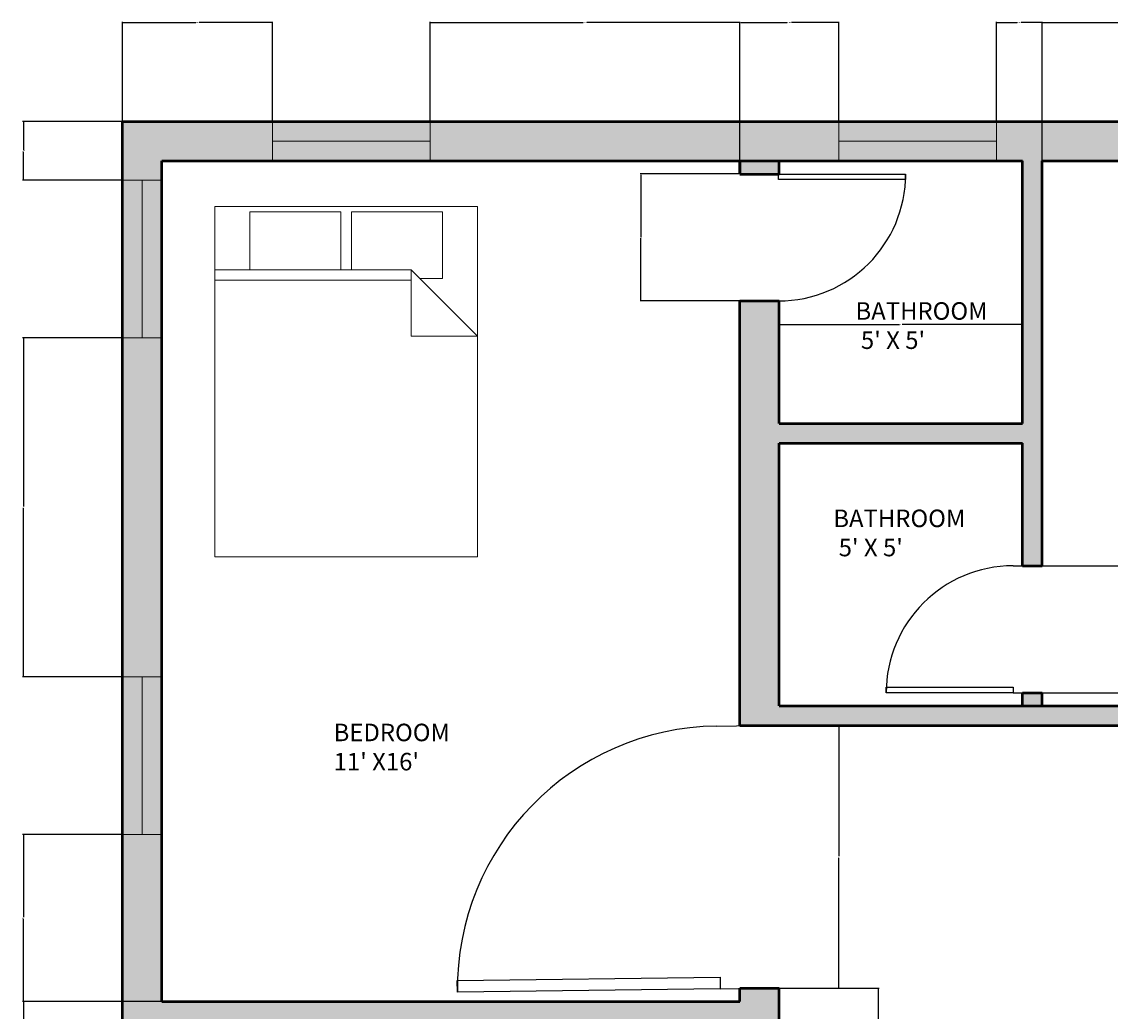
# Model space of a CAD drawing. Units: inches. Extents: x 7 to 493, y -11 to 454.
# Tile 2 of 4: x 7 to 255, y 228 to 454. Entities that reach past the tile are written whole.
import ezdxf

# ---------------------------------------------------------------- set-up
doc = ezdxf.new("R2010")
doc.units = ezdxf.units.IN
doc.header["$MEASUREMENT"] = 0
for name, color, linetype, lineweight in [('A-ANNO-DIMS', 2, 'Continuous', 18), ('A-AREA-IDEN', 7, 'Continuous', 25), ('A-WALL', 7, 'Continuous', 50), ('doors', 40, 'Continuous', 25), ('furniture', 220, 'Continuous', 18), ('window', 30, 'Continuous', 18)]:
    doc.layers.add(name, color=color, linetype=linetype, lineweight=lineweight)
doc.layers.add('A-WALL-PATT', color=251, linetype='Continuous', lineweight=13, true_color=0x636466)
doc.styles.get("Standard").update_dxf_attribs({"font": 'arial.ttf'})
doc.dimstyles.get("Standard").update_dxf_attribs({"dimtxt": 0.18, "dimasz": 0.18, "dimexe": 0.18, "dimexo": 0.0625, "dimgap": 0.09, "dimtad": 0, "dimtih": 1, "dimtoh": 1, "dimdec": 4, "dimzin": 0, "dimdsep": 46, "dimtxsty": 'Standard', "dimcen": 0.09, "dimadec": 0, "dimazin": 0, "dimtfac": 1, "dimtdec": 4, "dimtofl": 0, "dimtmove": 0, "dimatfit": 3, "dimfxl": 1, "dimtolj": 1, "dimtzin": 0, "dimarcsym": 0})

# ---------------------------------------------------------------- blocks, each defined once
blk = doc.blocks.new('Bed - Queen')
for p, q in [((0, -80.00003), (0, 0)), ((0, 0), (59.99999, 0)), ((59.99999, 0), (59.99999, -80.00003)), ((7.99999, -1.2), (28.79998, -1.2)), ((7.99999, -14.4), (7.99999, -1.2)), ((28.79998, -1.2), (28.79998, -14.4)), ((31.19999, -1.2), (51.99999, -1.2)), ((31.19999, -14.4), (31.19999, -1.2)), ((51.99999, -1.2), (51.99999, -16.4)), ((0, -14.4), (44.8, -14.4)), ((59.99999, -29.6), (44.8, -14.4)), ((44.8, -14.4), (44.8, -29.6)), ((44.8, -16.8), (0, -16.8)), ((51.99999, -16.4), (46.79936, -16.4)), ((44.8, -29.6), (59.99999, -29.6)), ((59.99999, -80.00003), (0, -80.00003))]:
    blk.add_line(p, q)
blk = doc.blocks.new('*U4')
for p, q in [((0, 0), (0, -6)), ((40, 0), (40, -6))]:
    blk.add_line(p, q)
blk.add_lwpolyline([(0, 0), (0, 40), (1.75, 40), (1.75, 0)], close=True)
blk.add_arc((0, 0), 40, 0, 90)
blk = doc.blocks.new('WIN-36IN')
for p, q in [((0, 0), (0, 9)), ((0, 9), (36, 9)), ((36, 9), (36, 0)), ((36, 9), (36, 4.5)), ((36, 4.5), (0, 4.5)), ((36, 0), (0, 0))]:
    blk.add_line(p, q)
blk = doc.blocks.new('*D24')
at = {"layer": 'A-ANNO-DIMS', "color": 0, "lineweight": -2, "transparency": 16777216}
for p, q in [((29.81, 431.55), (29.81, 454.27)), ((29.99, 454.09), (46.55, 454.09)), ((63.91, 454.09), (47.34, 454.09)), ((64.09, 431.55), (64.09, 454.27))]:
    blk.add_line(p, q, dxfattribs=at)
at = {"layer": 'A-ANNO-DIMS', "color": 0, "transparency": 16777216}
for points in [[(29.99, 454.12), (29.99, 454.06), (29.81, 454.09)], [(63.91, 454.12), (63.91, 454.06), (64.09, 454.09)]]:
    blk.add_solid(points, dxfattribs=at)
at = {"layer": 'Defpoints', "color": 0, "transparency": 16777216}
for p in [(64.09, 454.09), (29.81, 431.49), (64.09, 431.49)]:
    blk.add_point(p, dxfattribs=at)
at = {"layer": 'A-ANNO-DIMS', "color": 0, "transparency": 16777216, "insert": (46.95, 454.09), "char_height": 0.18, "attachment_point": 5}
blk.add_mtext('\\A1;34.28', dxfattribs=at)
blk = doc.blocks.new('*D25')
at = {"layer": 'A-ANNO-DIMS', "color": 0, "lineweight": -2, "transparency": 16777216}
for p, q in [((100.09, 431.55), (100.09, 454.27)), ((100.27, 454.09), (135.05, 454.09)), ((170.63, 454.09), (135.84, 454.09)), ((170.81, 422.55), (170.81, 454.27))]:
    blk.add_line(p, q, dxfattribs=at)
at = {"layer": 'A-ANNO-DIMS', "color": 0, "transparency": 16777216}
for points in [[(100.27, 454.12), (100.27, 454.06), (100.09, 454.09)], [(170.63, 454.12), (170.63, 454.06), (170.81, 454.09)]]:
    blk.add_solid(points, dxfattribs=at)
at = {"layer": 'Defpoints', "color": 0, "transparency": 16777216}
for p in [(170.81, 454.09), (100.09, 431.49), (170.81, 422.49)]:
    blk.add_point(p, dxfattribs=at)
at = {"layer": 'A-ANNO-DIMS', "color": 0, "transparency": 16777216, "insert": (135.45, 454.09), "char_height": 0.18, "attachment_point": 5}
blk.add_mtext('\\A1;70.72', dxfattribs=at)
blk = doc.blocks.new('*D26')
at = {"layer": 'A-ANNO-DIMS', "color": 0, "lineweight": -2, "transparency": 16777216}
for p, q in [((170.81, 422.55), (170.81, 454.27)), ((170.99, 454.09), (181.62, 454.09)), ((193.18, 454.09), (182.55, 454.09)), ((193.36, 431.55), (193.36, 454.27))]:
    blk.add_line(p, q, dxfattribs=at)
at = {"layer": 'A-ANNO-DIMS', "color": 0, "transparency": 16777216}
for points in [[(170.99, 454.12), (170.99, 454.06), (170.81, 454.09)], [(193.18, 454.12), (193.18, 454.06), (193.36, 454.09)]]:
    blk.add_solid(points, dxfattribs=at)
at = {"layer": 'Defpoints', "color": 0, "transparency": 16777216}
for p in [(193.36, 454.09), (193.36, 431.49), (170.81, 422.49)]:
    blk.add_point(p, dxfattribs=at)
at = {"layer": 'A-ANNO-DIMS', "color": 0, "transparency": 16777216, "insert": (182.08, 454.09), "char_height": 0.18, "attachment_point": 5}
blk.add_mtext('\\A1;22.553', dxfattribs=at)
blk = doc.blocks.new('*D27')
at = {"layer": 'A-ANNO-DIMS', "color": 0, "lineweight": -2, "transparency": 16777216}
for p, q in [((229.36, 431.55), (229.36, 454.27)), ((229.54, 454.09), (234.13, 454.09)), ((239.63, 454.09), (235.04, 454.09)), ((239.81, 422.55), (239.81, 454.27))]:
    blk.add_line(p, q, dxfattribs=at)
at = {"layer": 'A-ANNO-DIMS', "color": 0, "transparency": 16777216}
for points in [[(229.54, 454.12), (229.54, 454.06), (229.36, 454.09)], [(239.63, 454.12), (239.63, 454.06), (239.81, 454.09)]]:
    blk.add_solid(points, dxfattribs=at)
at = {"layer": 'Defpoints', "color": 0, "transparency": 16777216}
for p in [(239.81, 454.09), (229.36, 431.49), (239.81, 422.49)]:
    blk.add_point(p, dxfattribs=at)
at = {"layer": 'A-ANNO-DIMS', "color": 0, "transparency": 16777216, "insert": (234.58, 454.09), "char_height": 0.18, "attachment_point": 5}
blk.add_mtext('\\A1;10.447', dxfattribs=at)
blk = doc.blocks.new('*D28')
at = {"layer": 'A-ANNO-DIMS', "color": 0, "lineweight": -2, "transparency": 16777216}
for p, q in [((239.81, 422.55), (239.81, 454.27)), ((239.99, 454.09), (300.63, 454.09)), ((362.18, 454.09), (301.54, 454.09)), ((362.36, 431.55), (362.36, 454.27))]:
    blk.add_line(p, q, dxfattribs=at)
at = {"layer": 'A-ANNO-DIMS', "color": 0, "transparency": 16777216}
for points in [[(239.99, 454.12), (239.99, 454.06), (239.81, 454.09)], [(362.18, 454.12), (362.18, 454.06), (362.36, 454.09)]]:
    blk.add_solid(points, dxfattribs=at)
at = {"layer": 'Defpoints', "color": 0, "transparency": 16777216}
for p in [(362.36, 454.09), (362.36, 431.49), (239.81, 422.49)]:
    blk.add_point(p, dxfattribs=at)
at = {"layer": 'A-ANNO-DIMS', "color": 0, "transparency": 16777216, "insert": (301.08, 454.09), "char_height": 0.18, "attachment_point": 5}
blk.add_mtext('\\A1;122.55', dxfattribs=at)
blk = doc.blocks.new('*D33')
at = {"layer": 'A-ANNO-DIMS', "color": 0, "lineweight": -2, "transparency": 16777216}
for p, q in [((38.74, 230.49), (7.03, 230.49)), ((7.21, 230.31), (7.21, 216.31)), ((7.21, 201.94), (7.21, 215.94)), ((29.74, 201.76), (7.03, 201.76))]:
    blk.add_line(p, q, dxfattribs=at)
at = {"layer": 'A-ANNO-DIMS', "color": 0, "transparency": 16777216}
for points in [[(7.18, 230.31), (7.24, 230.31), (7.21, 230.49)], [(7.18, 201.94), (7.24, 201.94), (7.21, 201.76)]]:
    blk.add_solid(points, dxfattribs=at)
at = {"layer": 'Defpoints', "color": 0, "transparency": 16777216}
for p in [(7.21, 230.49), (38.81, 230.49), (29.81, 201.76)]:
    blk.add_point(p, dxfattribs=at)
at = {"layer": 'A-ANNO-DIMS', "color": 0, "transparency": 16777216, "insert": (7.21, 216.13), "char_height": 0.18, "attachment_point": 5}
blk.add_mtext('\\A1;28.72', dxfattribs=at)
blk = doc.blocks.new('*D34')
at = {"layer": 'A-ANNO-DIMS', "color": 0, "lineweight": -2, "transparency": 16777216}
for p, q in [((29.74, 268.63), (7.03, 268.63)), ((7.21, 268.45), (7.21, 249.74)), ((7.21, 230.67), (7.21, 249.37)), ((38.74, 230.49), (7.03, 230.49))]:
    blk.add_line(p, q, dxfattribs=at)
at = {"layer": 'A-ANNO-DIMS', "color": 0, "transparency": 16777216}
for points in [[(7.18, 268.45), (7.24, 268.45), (7.21, 268.63)], [(7.18, 230.67), (7.24, 230.67), (7.21, 230.49)]]:
    blk.add_solid(points, dxfattribs=at)
at = {"layer": 'Defpoints', "color": 0, "transparency": 16777216}
for p in [(7.21, 268.63), (29.81, 268.63), (38.81, 230.49)]:
    blk.add_point(p, dxfattribs=at)
at = {"layer": 'A-ANNO-DIMS', "color": 0, "transparency": 16777216, "insert": (7.21, 249.56), "char_height": 0.18, "attachment_point": 5}
blk.add_mtext('\\A1;38.14', dxfattribs=at)
blk = doc.blocks.new('*D35')
at = {"layer": 'A-ANNO-DIMS', "color": 0, "lineweight": -2, "transparency": 16777216}
for p, q in [((29.74, 382.06), (7.03, 382.06)), ((7.21, 381.88), (7.21, 343.53)), ((7.21, 304.81), (7.21, 343.16)), ((29.74, 304.63), (7.03, 304.63))]:
    blk.add_line(p, q, dxfattribs=at)
at = {"layer": 'A-ANNO-DIMS', "color": 0, "transparency": 16777216}
for points in [[(7.18, 381.88), (7.24, 381.88), (7.21, 382.06)], [(7.18, 304.81), (7.24, 304.81), (7.21, 304.63)]]:
    blk.add_solid(points, dxfattribs=at)
at = {"layer": 'Defpoints', "color": 0, "transparency": 16777216}
for p in [(7.21, 382.06), (29.81, 382.06), (29.81, 304.63)]:
    blk.add_point(p, dxfattribs=at)
at = {"layer": 'A-ANNO-DIMS', "color": 0, "transparency": 16777216, "insert": (7.21, 343.34), "char_height": 0.18, "attachment_point": 5}
blk.add_mtext('\\A1;77.43', dxfattribs=at)
blk = doc.blocks.new('*D36')
at = {"layer": 'A-ANNO-DIMS', "color": 0, "lineweight": -2, "transparency": 16777216}
for p, q in [((29.74, 431.49), (7.03, 431.49)), ((7.21, 431.31), (7.21, 424.95)), ((7.21, 418.24), (7.21, 424.59)), ((29.74, 418.06), (7.03, 418.06))]:
    blk.add_line(p, q, dxfattribs=at)
at = {"layer": 'A-ANNO-DIMS', "color": 0, "transparency": 16777216}
for points in [[(7.18, 431.31), (7.24, 431.31), (7.21, 431.49)], [(7.18, 418.24), (7.24, 418.24), (7.21, 418.06)]]:
    blk.add_solid(points, dxfattribs=at)
at = {"layer": 'Defpoints', "color": 0, "transparency": 16777216}
for p in [(7.21, 431.49), (29.81, 431.49), (29.81, 418.06)]:
    blk.add_point(p, dxfattribs=at)
at = {"layer": 'A-ANNO-DIMS', "color": 0, "transparency": 16777216, "insert": (7.21, 424.77), "char_height": 0.18, "attachment_point": 5}
blk.add_mtext('\\A1;13.427', dxfattribs=at)
blk = doc.blocks.new('*D51')
at = {"layer": 'A-ANNO-DIMS', "color": 0, "lineweight": -2, "transparency": 16777216}
for p, q in [((179.87, 233.49), (202.59, 233.49)), ((202.41, 233.31), (202.41, 213.38)), ((202.41, 193.1), (202.41, 213.02)), ((179.87, 192.92), (202.59, 192.92))]:
    blk.add_line(p, q, dxfattribs=at)
at = {"layer": 'A-ANNO-DIMS', "color": 0, "transparency": 16777216}
for points in [[(202.38, 233.31), (202.44, 233.31), (202.41, 233.49)], [(202.38, 193.1), (202.44, 193.1), (202.41, 192.92)]]:
    blk.add_solid(points, dxfattribs=at)
at = {"layer": 'Defpoints', "color": 0, "transparency": 16777216}
for p in [(179.81, 233.49), (179.81, 192.92), (202.41, 192.92)]:
    blk.add_point(p, dxfattribs=at)
at = {"layer": 'A-ANNO-DIMS', "color": 0, "transparency": 16777216, "insert": (202.41, 213.2), "char_height": 0.18, "attachment_point": 5}
blk.add_mtext('\\A1;40.57', dxfattribs=at)
blk = doc.blocks.new('*D55')
at = {"layer": 'A-ANNO-DIMS', "color": 0, "lineweight": -2, "transparency": 16777216}
for p, q in [((239.87, 329.99), (262.59, 329.99)), ((262.41, 329.81), (262.41, 315.67)), ((262.41, 301.17), (262.41, 315.3)), ((239.87, 300.99), (262.59, 300.99))]:
    blk.add_line(p, q, dxfattribs=at)
at = {"layer": 'A-ANNO-DIMS', "color": 0, "transparency": 16777216}
for points in [[(262.38, 329.81), (262.44, 329.81), (262.41, 329.99)], [(262.38, 301.17), (262.44, 301.17), (262.41, 300.99)]]:
    blk.add_solid(points, dxfattribs=at)
at = {"layer": 'Defpoints', "color": 0, "transparency": 16777216}
for p in [(239.81, 329.99), (239.81, 300.99), (262.41, 300.99)]:
    blk.add_point(p, dxfattribs=at)
at = {"layer": 'A-ANNO-DIMS', "color": 0, "transparency": 16777216, "insert": (262.41, 315.49), "char_height": 0.18, "attachment_point": 5}
blk.add_mtext('\\A1;29', dxfattribs=at)
blk = doc.blocks.new('*D56')
at = {"layer": 'A-ANNO-DIMS', "color": 0, "lineweight": -2, "transparency": 16777216}
for p, q in [((170.87, 293.49), (193.59, 293.49)), ((193.41, 293.31), (193.41, 263.67)), ((193.41, 233.67), (193.41, 263.3)), ((170.87, 233.49), (193.59, 233.49))]:
    blk.add_line(p, q, dxfattribs=at)
at = {"layer": 'A-ANNO-DIMS', "color": 0, "transparency": 16777216}
for points in [[(193.38, 293.31), (193.44, 293.31), (193.41, 293.49)], [(193.38, 233.67), (193.44, 233.67), (193.41, 233.49)]]:
    blk.add_solid(points, dxfattribs=at)
at = {"layer": 'Defpoints', "color": 0, "transparency": 16777216}
for p in [(170.81, 293.49), (170.81, 233.49), (193.41, 233.49)]:
    blk.add_point(p, dxfattribs=at)
at = {"layer": 'A-ANNO-DIMS', "color": 0, "transparency": 16777216, "insert": (193.41, 263.49), "char_height": 0.18, "attachment_point": 5}
blk.add_mtext('\\A1;60', dxfattribs=at)
blk = doc.blocks.new('*D57')
at = {"layer": 'A-ANNO-DIMS', "color": 0, "lineweight": -2, "transparency": 16777216}
for p, q in [((170.74, 419.49), (148.03, 419.49)), ((148.21, 419.31), (148.21, 405.17)), ((148.21, 390.67), (148.21, 404.8)), ((170.74, 390.49), (148.03, 390.49))]:
    blk.add_line(p, q, dxfattribs=at)
at = {"layer": 'A-ANNO-DIMS', "color": 0, "transparency": 16777216}
for points in [[(148.18, 419.31), (148.24, 419.31), (148.21, 419.49)], [(148.18, 390.67), (148.24, 390.67), (148.21, 390.49)]]:
    blk.add_solid(points, dxfattribs=at)
at = {"layer": 'Defpoints', "color": 0, "transparency": 16777216}
for p in [(148.21, 419.49), (170.81, 419.49), (170.81, 390.49)]:
    blk.add_point(p, dxfattribs=at)
at = {"layer": 'A-ANNO-DIMS', "color": 0, "transparency": 16777216, "insert": (148.21, 404.99), "char_height": 0.18, "attachment_point": 5}
blk.add_mtext('\\A1;29', dxfattribs=at)
blk = doc.blocks.new('*D58')
at = {"layer": 'A-ANNO-DIMS', "color": 0, "lineweight": -2, "transparency": 16777216}
for p, q in [((179.81, 362.55), (179.81, 385.27)), ((235.31, 362.55), (235.31, 385.27)), ((179.99, 385.09), (207.23, 385.09)), ((235.13, 385.09), (207.88, 385.09))]:
    blk.add_line(p, q, dxfattribs=at)
at = {"layer": 'A-ANNO-DIMS', "color": 0, "transparency": 16777216}
for points in [[(179.99, 385.12), (179.99, 385.06), (179.81, 385.09)], [(235.13, 385.12), (235.13, 385.06), (235.31, 385.09)]]:
    blk.add_solid(points, dxfattribs=at)
at = {"layer": 'Defpoints', "color": 0, "transparency": 16777216}
for p in [(235.31, 385.09), (179.81, 362.49), (235.31, 362.49)]:
    blk.add_point(p, dxfattribs=at)
at = {"layer": 'A-ANNO-DIMS', "color": 0, "transparency": 16777216, "insert": (207.56, 385.09), "char_height": 0.18, "attachment_point": 5}
blk.add_mtext('\\A1;55.5', dxfattribs=at)

msp = doc.modelspace()

# ---------------------------------------------------------------- hatches: boundary and pattern name
at = {"layer": 'A-WALL-PATT'}
h = msp.add_hatch(color=256, dxfattribs=at)
h.dxf.hatch_style = 1
h.paths.add_polyline_path([(29.8054, 11.4863), (449.8054, 11.4863), (449.8054, 431.4863), (29.8054, 431.4863)])
h.paths.add_polyline_path([(38.8054, 422.4863), (235.3054, 422.4863), (235.3054, 362.4863), (179.8054, 362.4863), (179.8054, 390.4863), (170.8054, 390.4863), (170.8054, 293.4863), (353.0513, 293.4863), (353.0513, 297.9863), (239.8054, 297.9863), (235.3054, 297.9863), (179.8054, 297.9863), (179.8054, 357.9863), (235.3054, 357.9863), (235.3054, 329.9863), (239.8054, 329.9863), (239.8054, 422.4863), (440.8054, 422.4863), (440.8054, 297.9863), (413.0513, 297.9863), (413.0513, 293.4863), (440.8054, 293.4863), (440.8054, 110.4863), (402.7135, 110.4863), (402.7135, 101.5532), (402.7135, 101.4863), (440.8054, 101.4863), (440.8054, 20.4863), (179.8054, 20.4863), (179.8054, 101.4863), (255.3658, 101.4863), (255.3658, 110.4863), (179.8054, 110.4863), (179.8054, 146.9794), (170.8054, 146.9794), (170.8054, 20.4863), (117.9037, 20.4863), (117.9037, 15.9863), (81.9037, 15.9863), (81.9037, 20.4863), (38.8054, 20.4863), (38.8054, 125.4863), (118.4942, 125.4863), (118.4942, 129.9863), (38.8054, 129.9863), (38.8054, 225.9863), (170.8054, 225.9863), (170.8054, 192.9161), (179.8054, 192.9161), (179.8054, 233.4863), (170.8054, 233.4863), (170.8054, 230.4863), (38.8054, 230.4863)], flags=16)
h.paths.add_polyline_path([(53.2938, 207.1427), (65.8095, 207.1427), (67.0594, 215.1427), (83.5282, 215.1427), (84.7782, 207.1427), (93.8095, 207.1427), (95.0594, 215.1427), (111.5282, 215.1427), (112.7782, 207.1427), (125.2938, 207.1427), (125.2938, 198.6271), (133.2938, 197.3771), (133.2938, 180.9083), (125.2938, 179.6583), (125.2938, 171.1427), (112.7782, 171.1427), (111.5282, 163.1427), (95.0594, 163.1427), (93.8095, 171.1427), (84.7782, 171.1427), (83.5282, 163.1427), (67.0594, 163.1427), (65.8095, 171.1427), (53.2938, 171.1427), (53.2938, 179.6583), (45.2938, 180.9083), (45.2938, 197.3771), (53.2938, 198.6271)], flags=0)
h.paths.add_polyline_path([(98.6154, 202.5867), (98.6833, 202.7415), (98.7209, 202.9031), (98.7311, 203.0686), (98.717, 203.2352), (98.6813, 203.3997), (98.6271, 203.5594), (98.5576, 203.7119), (98.4774, 203.8575), (98.3913, 203.9974), (98.2332, 204.2423), (98.1033, 204.4662), (98.0223, 204.7063), (98.0302, 204.9526), (98.1325, 205.1802), (98.329, 205.372), (98.3993, 205.406), (98.2782, 205.3224), (98.1805, 205.227), (98.1063, 205.1219), (98.0555, 205.0089), (98.0282, 204.8901), (98.0243, 204.7674), (98.0438, 204.6427), (98.086, 204.5175), (98.1467, 204.3914), (98.221, 204.2633), (98.3042, 204.1323), (98.4533, 203.9013), (98.6038, 203.6279), (98.7103, 203.3143), (98.7386, 202.9794), (98.6633, 202.6554)], flags=0)
h.paths.add_polyline_path([(67.2938, 216.6427), (83.2938, 216.6427), (83.45, 215.6427), (67.1375, 215.6427)], flags=0)
h.paths.add_polyline_path([(43.7938, 197.1427), (44.7938, 197.2989), (44.7938, 180.9864), (43.7938, 181.1427)], flags=0)
h.paths.add_polyline_path([(106.3833, 198.8302), (106.2808, 199.0177), (106.1587, 199.2052), (106.023, 199.3927), (105.8794, 199.5802), (105.6298, 199.9018), (105.4605, 200.1427), (105.3438, 200.33), (105.1938, 200.6147), (105.0892, 200.9776), (105.1, 201.3227), (105.1358, 201.3994), (105.0972, 201.2325), (105.0918, 201.0599), (105.1167, 200.8823), (105.169, 200.7008), (105.2456, 200.5164), (105.3438, 200.33), (105.4605, 200.1427), (105.5923, 199.9552), (105.7339, 199.7677), (105.8794, 199.5802), (106.1138, 199.2741), (106.3496, 198.9121)], flags=0)
h.paths.add_polyline_path([(124.5037, 189.2544), (124.6786, 189.213), (124.7978, 189.1834), (124.8824, 189.1635), (124.9532, 189.1515), (125.0583, 189.1432), (125.138, 189.143), (124.9529, 189.147), (124.7978, 189.1834), (124.5749, 189.2388)], flags=0)
h.paths.add_polyline_path([(95.2938, 216.6427), (111.2938, 216.6427), (111.45, 215.6427), (95.1375, 215.6427)], flags=0)
h.paths.add_polyline_path([(191.6785, 332.1221), (224.065, 332.1221), (224.065, 343.8649), (191.6785, 343.8649)], flags=8)
h.paths.add_polyline_path([(196.7522, 379.4931), (229.1387, 379.4931), (229.1387, 391.2359), (196.7522, 391.2359)], flags=8)
h.paths.add_polyline_path([(232.397, 56.3062), (260.115, 56.3062), (260.115, 68.0654), (232.397, 68.0654)], flags=8)
h.paths.add_polyline_path([(90.1783, 70.3293), (134.3492, 70.3293), (134.3492, 82.0885), (90.1783, 82.0885)], flags=8)
h.paths.add_polyline_path([(126.7274, 208.2711), (165.9297, 208.2711), (165.9297, 220.0303), (126.7274, 220.0303)], flags=8)
h.paths.add_polyline_path([(261.4741, 205.6105), (297.4786, 205.6105), (297.4786, 217.3697), (261.4741, 217.3697)], flags=8)
h.paths.add_polyline_path([(77.3838, 283.1969), (106.5561, 283.1969), (106.5561, 294.9561), (77.3838, 294.9561)], flags=8)
h.paths.add_polyline_path([(357.5163, 353.5423), (386.6886, 353.5423), (386.6886, 365.3015), (357.5163, 365.3015)], flags=8)
h = msp.add_hatch(color=256, dxfattribs=at)
h.dxf.hatch_style = 1
h.paths.add_polyline_path([(179.8054, 422.4863), (170.8054, 422.4863), (170.8054, 419.4863), (179.8054, 419.4863)])
h = msp.add_hatch(color=256, dxfattribs=at)
h.dxf.hatch_style = 1
h.paths.add_polyline_path([(239.8054, 300.9863), (235.3054, 300.9863), (235.3054, 297.9863), (239.8054, 297.9863)])

# ---------------------------------------------------------------- linework, layer by layer
at = {"layer": 'A-WALL'}
for p, q in [((38.8054, 422.4863), (235.3054, 422.4863)), ((38.8054, 230.4863), (38.8054, 422.4863)), ((170.8054, 419.4863), (170.8054, 422.4863)), ((170.8054, 422.4863), (170.8054, 419.4863)), ((179.8054, 419.4863), (179.8054, 422.4863)), ((179.8054, 419.4863), (179.8054, 422.4863)), ((235.3054, 362.4863), (235.3054, 422.4863)), ((239.8054, 422.4863), (440.8054, 422.4863)), ((239.8054, 329.9863), (239.8054, 422.4863)), ((170.8054, 419.4863), (179.8054, 419.4863)), ((170.8054, 293.4863), (170.8054, 390.4863)), ((170.8054, 390.4863), (179.8054, 390.4863)), ((179.8054, 362.4863), (179.8054, 390.4863)), ((179.8054, 362.4863), (235.3054, 362.4863)), ((179.8054, 357.9863), (235.3054, 357.9863)), ((179.8054, 297.9863), (179.8054, 357.9863)), ((235.3054, 329.9863), (235.3054, 357.9863)), ((235.3054, 329.9863), (239.8054, 329.9863)), ((235.3054, 300.9863), (239.8054, 300.9863)), ((235.3054, 297.9863), (235.3054, 300.9863)), ((239.8054, 297.9863), (239.8054, 300.9863)), ((179.8054, 297.9863), (235.3054, 297.9863)), ((235.3054, 297.9863), (239.8054, 297.9863)), ((239.8054, 297.9863), (353.0513, 297.9863)), ((170.8054, 293.4863), (353.0513, 293.4863)), ((170.8054, 233.4863), (179.8054, 233.4863)), ((170.8054, 230.4863), (170.8054, 233.4863)), ((179.8054, 192.9161), (179.8054, 233.4863)), ((38.8054, 230.4863), (170.8054, 230.4863))]:
    msp.add_line(p, q, dxfattribs=at)
msp.add_lwpolyline([(29.8054, 431.4863), (449.8054, 431.4863), (449.8054, 11.4863), (29.8054, 11.4863)], close=True, dxfattribs=at)

# ---------------------------------------------------------------- block references
at = {"layer": 'doors'}
for p, xscale, yscale, zscale, rotation in [((179.6554, 419.4863), 0.7249999999999993, 0.7249999999999993, 0.7249999999999993, 270), ((233.2054, 300.9863), 0.7249999999999993, 0.7249999999999993, 0.7249999999999993, 90.00000000002335), ((166.3054, 233.3709), 1.500123303159216, 1.500123303159216, 1.500123303159216, 90.73462250426493)]:
    msp.add_blockref('*U4', p, dxfattribs=dict(at, xscale=xscale, yscale=yscale, zscale=zscale, rotation=rotation))
at = {"layer": 'furniture'}
msp.add_blockref('Bed - Queen', (50.9129, 412.0336), dxfattribs=at)
at = {"layer": 'window'}
for p in [(64.0857, 422.486), (193.359, 422.486)]:
    msp.add_blockref('WIN-36IN', p, dxfattribs=at)
at = {"layer": 'window', "extrusion": (0, 0, -1), "zscale": -1, "rotation": 269.9999999999984}
for p in [(-38.8057, 418.0591), (-38.8057, 304.627)]:
    msp.add_blockref('WIN-36IN', p, dxfattribs=at)

# ---------------------------------------------------------------- texts
at = {"layer": 'A-AREA-IDEN', "char_height": 0.2, "attachment_point": 1}
for s, insert in [("{\\H20x;BATHROOM\\P 5' X 5'}", (197.2115, 390.1982)), ("{\\H20x;BATHROOM\\P 5' X 5'}", (192.1377, 342.8272)), ("{\\H20x;BEDROOM\\P11' X16'}", (78.0423, 293.9184))]:
    msp.add_mtext_dynamic_manual_height_columns(s, width=58.591086, gutter_width=1, heights=[0], dxfattribs=dict(at, insert=insert))

# ---------------------------------------------------------------- dimensions: what is measured, and where the dimension line sits
at = {"layer": 'A-ANNO-DIMS'}
for base, p1, p2, override, picture, middle in [((64.0855, 454.0863), (29.8054, 431.4863), (64.0855, 431.4863), {"dimdec": 2, "dimlfac": 1, "dimrnd": 0, "dimzin": 0, "dimdsep": 46, "dimlunit": 2}, '*D24', (46.9454, 454.0863)), ((170.8054, 454.0863), (100.0855, 431.4863), (170.8054, 422.4863), {"dimdec": 2, "dimlfac": 1, "dimrnd": 0, "dimzin": 0, "dimdsep": 46, "dimlunit": 2}, '*D25', (135.4454, 454.0863)), ((193.3588, 454.0863), (170.8054, 422.4863), (193.3588, 431.4863), {"dimdec": 3, "dimlfac": 1, "dimrnd": 0, "dimzin": 0, "dimdsep": 46, "dimlunit": 2}, '*D26', (182.0821, 454.0863)), ((239.8054, 454.0863), (229.3588, 431.4863), (239.8054, 422.4863), {"dimdec": 3, "dimlfac": 1, "dimrnd": 0, "dimzin": 0, "dimdsep": 46, "dimlunit": 2}, '*D27', (234.5821, 454.0863)), ((362.3579, 454.0863), (239.8054, 422.4863), (362.3579, 431.4863), {"dimdec": 2, "dimlfac": 1, "dimrnd": 0, "dimzin": 0, "dimdsep": 46, "dimlunit": 2}, '*D28', (301.0816, 454.0863)), ((235.3054, 385.0863), (179.8054, 362.4863), (235.3054, 362.4863), {"dimdec": 1, "dimlfac": 1, "dimrnd": 0, "dimzin": 0, "dimdsep": 46, "dimlunit": 2}, '*D58', (207.5554, 385.0863))]:
    dim = msp.add_linear_dim(base=base, p1=p1, p2=p2, dimstyle='Standard', override=override, dxfattribs=at)
    dim.commit()
    dim.dimension.update_dxf_attribs({"geometry": picture, "text_midpoint": middle})
for base, p1, p2, angle, override, picture, middle in [((7.2054, 431.4863), (29.8054, 418.0593), (29.8054, 431.4863), 90, {"dimdec": 3, "dimlfac": 1, "dimrnd": 0, "dimzin": 0, "dimdsep": 46, "dimlunit": 2}, '*D36', (7.2054, 424.7728)), ((148.2054, 419.4863), (170.8054, 390.4863), (170.8054, 419.4863), 90, {"dimdec": 0, "dimlfac": 1, "dimrnd": 0, "dimzin": 0, "dimdsep": 46, "dimlunit": 2}, '*D57', (148.2054, 404.9863)), ((7.2054, 382.0593), (29.8054, 304.6272), (29.8054, 382.0593), 90, {"dimdec": 2, "dimlfac": 1, "dimrnd": 0, "dimzin": 0, "dimdsep": 46, "dimlunit": 2}, '*D35', (7.2054, 343.3432)), ((262.4054, 300.9863), (239.8054, 329.9863), (239.8054, 300.9863), 270, {"dimdec": 0, "dimlfac": 1, "dimrnd": 0, "dimzin": 0, "dimdsep": 46, "dimlunit": 2}, '*D55', (262.4054, 315.4863)), ((193.4054, 233.4863), (170.8054, 293.4863), (170.8054, 233.4863), 270, {"dimdec": 0, "dimlfac": 1, "dimrnd": 0, "dimzin": 0, "dimdsep": 46, "dimlunit": 2}, '*D56', (193.4054, 263.4863)), ((7.2054, 268.6272), (38.8054, 230.4863), (29.8054, 268.6272), 90, {"dimdec": 2, "dimlfac": 1, "dimrnd": 0, "dimzin": 0, "dimdsep": 46, "dimlunit": 2}, '*D34', (7.2054, 249.5568)), ((202.4054, 192.9161), (179.8054, 233.4863), (179.8054, 192.9161), 270, {"dimdec": 2, "dimlfac": 1, "dimrnd": 0, "dimzin": 0, "dimdsep": 46, "dimlunit": 2}, '*D51', (202.4054, 213.2012)), ((7.2054, 230.4863), (29.8054, 201.764), (38.8054, 230.4863), 90, {"dimdec": 2, "dimlfac": 1, "dimrnd": 0, "dimzin": 0, "dimdsep": 46, "dimlunit": 2}, '*D33', (7.2054, 216.1252))]:
    dim = msp.add_linear_dim(base=base, p1=p1, p2=p2, angle=angle, dimstyle='Standard', override=override, dxfattribs=at)
    dim.commit()
    dim.dimension.update_dxf_attribs({"geometry": picture, "text_midpoint": middle})

doc.saveas('drawing.dxf')
